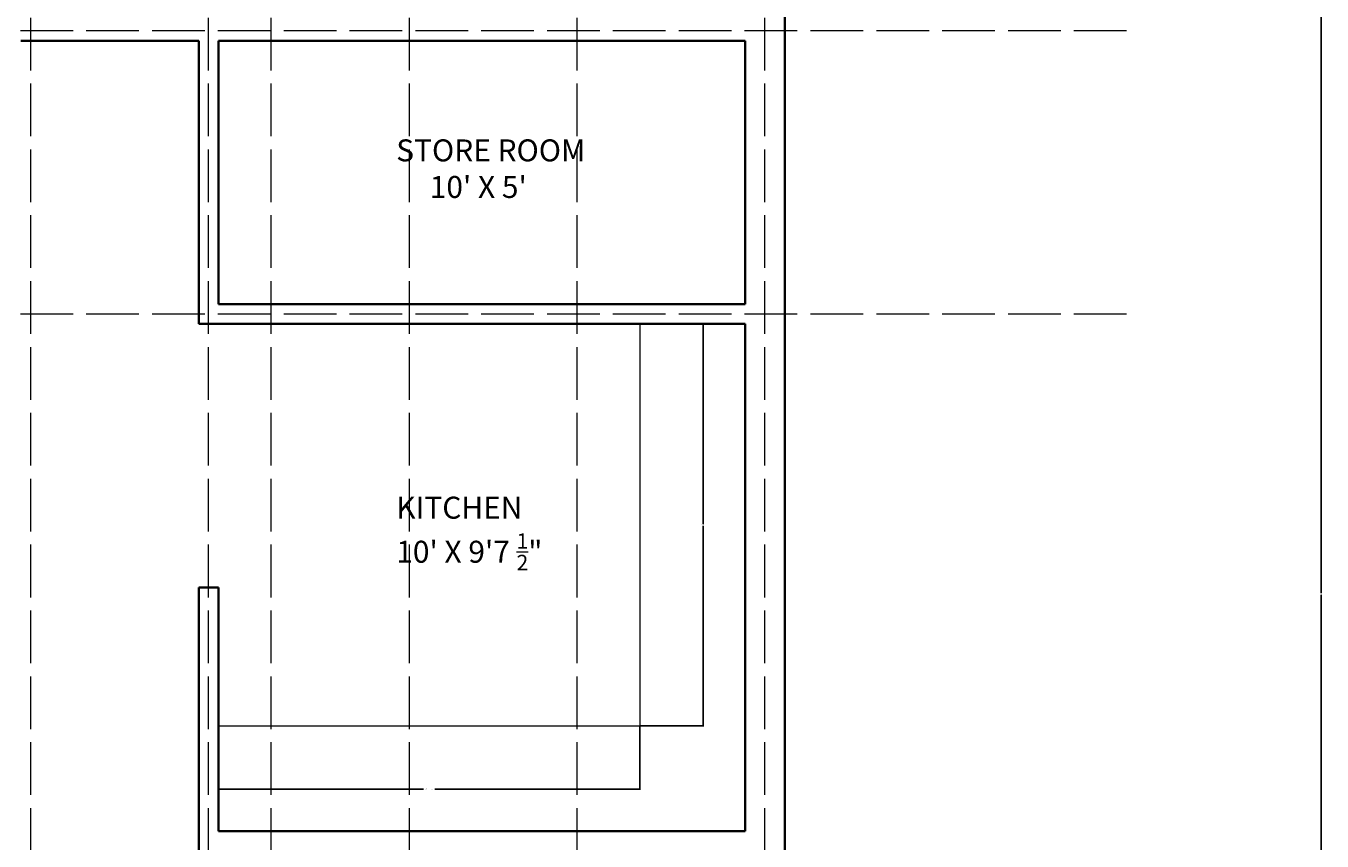
# Model space of a CAD drawing. Units: inches. Extents: x 1159 to 4240, y 1112 to 2085.
# Tile 8 of 13: x 1535 to 1831, y 1551 to 1737. Entities that reach past the tile are written whole.
import ezdxf

# ---------------------------------------------------------------- set-up
doc = ezdxf.new("R2010")
doc.units = ezdxf.units.IN
doc.linetypes.add('ACAD_ISO02W100', pattern=[15, 12, -3])
for name, color, linetype, lineweight in [('A-ANNO-DIMS', 2, 'Continuous', 18), ('A-AREA-IDEN', 30, 'Continuous', 18), ('A-GRID', 8, 'ACAD_ISO02W100', 13), ('KITCHEN', 1, 'Continuous', 18), ('WALL', 7, 'Continuous', 35)]:
    doc.layers.add(name, color=color, linetype=linetype, lineweight=lineweight)
doc.styles.get("Standard").update_dxf_attribs({"font": 'arial.ttf'})
doc.dimstyles.get("Standard").update_dxf_attribs({"dimtxt": 0.18, "dimasz": 0.18, "dimexe": 0.18, "dimexo": 0.0625, "dimgap": 0.09, "dimtad": 0, "dimtih": 1, "dimtoh": 1, "dimdec": 4, "dimzin": 0, "dimdsep": 46, "dimtxsty": 'Standard', "dimcen": 0.09, "dimadec": 0, "dimazin": 0, "dimtfac": 1, "dimtdec": 4, "dimtofl": 0, "dimtmove": 0, "dimatfit": 3, "dimfxl": 1, "dimtolj": 1, "dimtzin": 0, "dimarcsym": 0})

# ---------------------------------------------------------------- blocks, each defined once
blk = doc.blocks.new('HOUSE-35x60-WALL-LAYOUT')
for p, q in [((420, 720), (420, 297)), ((246, 486), (286.5, 486)), ((286.5, 486), (286.5, 421.5)), ((291, 486), (291, 426)), ((291, 486), (411, 486)), ((411, 486), (411, 426)), ((291, 426), (411, 426)), ((291, 421.5), (286.5, 421.5)), ((291, 421.5), (411, 421.5)), ((411, 421.5), (411, 306)), ((291, 361.5), (286.5, 361.5)), ((286.5, 361.5), (286.5, 297)), ((291, 361.5), (291, 306)), ((291, 306), (411, 306))]:
    blk.add_line(p, q)
blk = doc.blocks.new('KITCHEN-COUNTER-L')
for p in [(96, 91.5), (0, 0)]:
    blk.add_line(p, (96, 0))
blk = doc.blocks.new('HOUSE-35x60-SETTING-OUT-GRID')
for p, q in [((333.07, 0), (333.07, 883.25)), ((373.57, 0), (373.57, 883.25)), ((387.82, 0), (387.82, 883.25)), ((419.32, 0), (419.32, 883.25)), ((457.57, 0), (457.57, 883.25)), ((500.32, 0), (500.32, 883.25)), ((582.7, 579), (0, 579)), ((582.7, 514.5), (0, 514.5))]:
    blk.add_line(p, q)
blk = doc.blocks.new('*D10')
at = {"layer": 'A-ANNO-DIMS', "color": 0, "lineweight": -2, "transparency": 16777216}
for p, q in [((1579.13, 1577.64), (1579.13, 1563.12)), ((1675.13, 1577.64), (1675.13, 1563.12)), ((1579.31, 1563.3), (1625.83, 1563.3)), ((1674.95, 1563.3), (1628.42, 1563.3))]:
    blk.add_line(p, q, dxfattribs=at)
at = {"layer": 'A-ANNO-DIMS', "color": 0, "lineweight": 100, "transparency": 16777216}
for points in [[(1579.31, 1563.33), (1579.31, 1563.27), (1579.13, 1563.3)], [(1674.95, 1563.33), (1674.95, 1563.27), (1675.13, 1563.3)]]:
    blk.add_solid(points, dxfattribs=at)
at = {"layer": 'Defpoints', "color": 0, "lineweight": 100, "transparency": 16777216}
for p in [(1579.13, 1577.7), (1675.13, 1577.7), (1675.13, 1563.3)]:
    blk.add_point(p, dxfattribs=at)
at = {"layer": 'A-ANNO-DIMS', "color": 0, "transparency": 16777216, "insert": (1627.13, 1563.3), "char_height": 0.18, "attachment_point": 5}
blk.add_mtext('\\A1;L-COUNTER 96 TYP.', dxfattribs=at)
blk = doc.blocks.new('*D11')
at = {"layer": 'A-ANNO-DIMS', "color": 0, "lineweight": -2, "transparency": 16777216}
for p, q in [((1675.19, 1669.2), (1689.71, 1669.2)), ((1689.53, 1669.02), (1689.53, 1623.63)), ((1689.53, 1577.88), (1689.53, 1623.27)), ((1675.19, 1577.7), (1689.71, 1577.7))]:
    blk.add_line(p, q, dxfattribs=at)
at = {"layer": 'A-ANNO-DIMS', "color": 0, "lineweight": 100, "transparency": 16777216}
for points in [[(1689.5, 1669.02), (1689.56, 1669.02), (1689.53, 1669.2)], [(1689.5, 1577.88), (1689.56, 1577.88), (1689.53, 1577.7)]]:
    blk.add_solid(points, dxfattribs=at)
at = {"layer": 'Defpoints', "color": 0, "lineweight": 100, "transparency": 16777216}
for p in [(1675.13, 1669.2), (1689.53, 1669.2), (1675.13, 1577.7)]:
    blk.add_point(p, dxfattribs=at)
at = {"layer": 'A-ANNO-DIMS', "color": 0, "transparency": 16777216, "insert": (1689.53, 1623.45), "char_height": 0.18, "attachment_point": 5}
blk.add_mtext('\\A1;92 TYP.', dxfattribs=at)
blk = doc.blocks.new('*D23')
at = {"layer": 'A-ANNO-DIMS', "color": 0, "lineweight": -2, "transparency": 16777216}
for p, q in [((1708.19, 1967.7), (1830.54, 1967.7)), ((1830.36, 1967.52), (1830.36, 1607.88)), ((1830.36, 1247.88), (1830.36, 1607.52)), ((1708.19, 1247.7), (1830.54, 1247.7))]:
    blk.add_line(p, q, dxfattribs=at)
at = {"layer": 'A-ANNO-DIMS', "color": 0, "lineweight": 100, "transparency": 16777216}
for points in [[(1830.33, 1967.52), (1830.39, 1967.52), (1830.36, 1967.7)], [(1830.33, 1247.88), (1830.39, 1247.88), (1830.36, 1247.7)]]:
    blk.add_solid(points, dxfattribs=at)
at = {"layer": 'Defpoints', "color": 0, "lineweight": 100, "transparency": 16777216}
for p in [(1708.13, 1967.7), (1830.36, 1967.7), (1708.13, 1247.7)]:
    blk.add_point(p, dxfattribs=at)
at = {"layer": 'A-ANNO-DIMS', "color": 0, "transparency": 16777216, "insert": (1830.36, 1607.7), "char_height": 0.18, "attachment_point": 5}
blk.add_mtext('\\A1;720', dxfattribs=at)

msp = doc.modelspace()

# ---------------------------------------------------------------- block references
at = {"layer": 'A-GRID'}
msp.add_blockref('HOUSE-35x60-SETTING-OUT-GRID', (1203.31, 1156.954), dxfattribs=at)
at = {"layer": 'KITCHEN'}
msp.add_blockref('KITCHEN-COUNTER-L', (1579.126, 1577.702), dxfattribs=at)
at = {"layer": 'WALL'}
msp.add_blockref('HOUSE-35x60-WALL-LAYOUT', (1288.126, 1247.702), dxfattribs=at)

# ---------------------------------------------------------------- texts
at = {"layer": 'A-AREA-IDEN', "char_height": 5, "attachment_point": 1}
for s, insert in [("\\A1;STORE ROOM\\P     10' X 5'", (1619.62, 1711.241)), ('\\A1;KITCHEN\\P10\' X 9\'7 {\\H0.7x;\\S1/2;}"', (1619.62, 1629.873))]:
    msp.add_mtext_dynamic_manual_height_columns(s, width=140.18614, gutter_width=12.5, heights=[0], dxfattribs=dict(at, insert=insert))

# ---------------------------------------------------------------- dimensions: what is measured, and where the dimension line sits
at = {"layer": 'A-ANNO-DIMS'}
dim = msp.add_linear_dim(base=(1830.364, 1967.702), p1=(1708.125, 1247.702), p2=(1708.125, 1967.702), angle=90, dimstyle='Standard', override={"dimdec": 0, "dimlfac": 1, "dimrnd": 0, "dimzin": 0, "dimdsep": 46, "dimlunit": 2}, dxfattribs=at)
dim.commit()
dim.dimension.update_dxf_attribs({"geometry": '*D23', "text_midpoint": (1830.364, 1607.702)})
dim = msp.add_linear_dim(base=(1689.525453697, 1669.201978604), p1=(1675.125453697, 1577.701978604), p2=(1675.125453697, 1669.201978604), angle=90, text='<> TYP.', dimstyle='Standard', override={"dimdec": 0, "dimlfac": 1, "dimrnd": 0, "dimzin": 0, "dimdsep": 46, "dimlunit": 2}, dxfattribs=at)
dim.commit()
dim.dimension.update_dxf_attribs({"geometry": '*D11', "text_midpoint": (1689.525453697, 1623.451978604)})
dim = msp.add_linear_dim(base=(1675.125, 1563.302), p1=(1579.125, 1577.702), p2=(1675.125, 1577.702), text='L-COUNTER <> TYP.', dimstyle='Standard', override={"dimdec": 0, "dimlfac": 1, "dimrnd": 0, "dimzin": 0, "dimdsep": 46, "dimlunit": 2}, dxfattribs=at)
dim.commit()
dim.dimension.update_dxf_attribs({"geometry": '*D10', "text_midpoint": (1627.125, 1563.302)})

doc.saveas('drawing.dxf')
